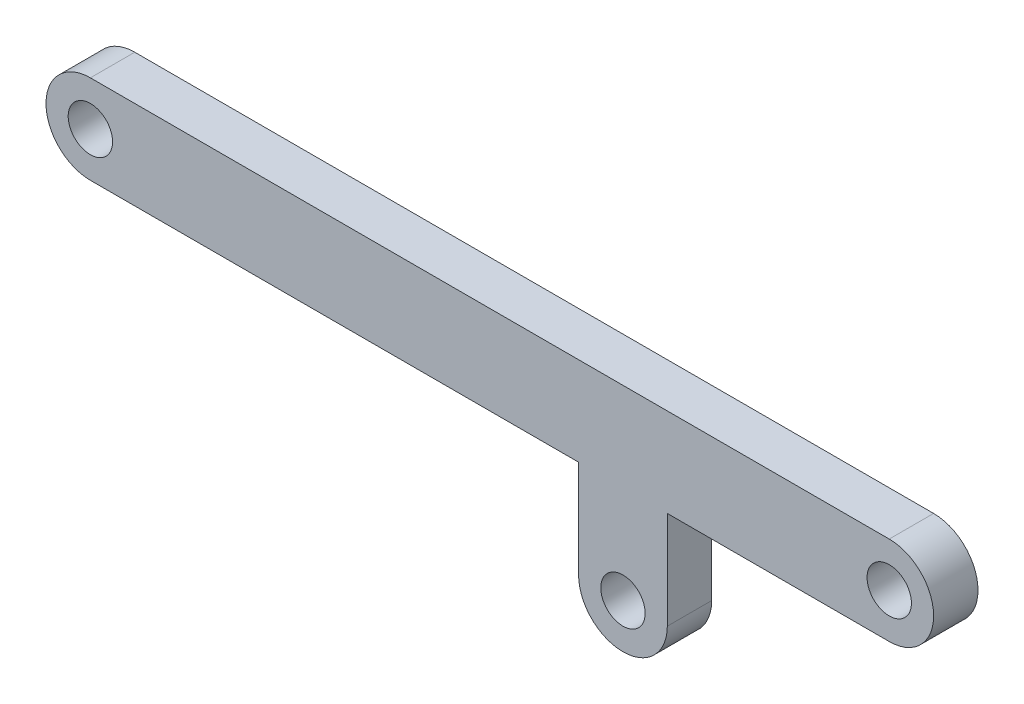
SolidWorks part; units mm, degrees
material "Plain Carbon Steel"
ref_plane "Front Plane" through (0, 0, 0) normal (0, 0, 1) x (1, 0, 0)
ref_plane "Top Plane" through (0, 0, 0) normal (0, 1, 0) x (1, 0, 0)
ref_plane "Right Plane" through (0, 0, 0) normal (1, 0, 0) x (0, 0, -1)
sketch "Link Plate Profile" plane through (0, 0, 0) normal (0, 0, 1) x (1, 0, 0)
  line L0 (45, 0) -> (-45, 0) construction
  line L1 (45, -5) -> (-45, -5)
  line L2 (45, 5) -> (-45, 5)
  line L3 (15, 6) -> (15, -16) construction
  line L4 (20, 6) -> (20, -16)
  line L5 (10, 6) -> (10, -16)
  arc A0 (45, -5) -> (45, 5) centre (45, 0) ccw
  arc A1 (-45, 5) -> (-45, -5) centre (-45, 0) ccw
  arc A2 (20, 6) -> (10, 6) centre (15, 6) ccw
  arc A3 (10, -16) -> (20, -16) centre (15, -16) ccw
  circle A4 centre (-45, 0) radius 2.5
  circle A5 centre (45, 0) radius 2.5
  circle A6 centre (15, -16) radius 2.5
  point P2 (0, 0)
  point P9 (15, -5)
  dimension "D1" = 5
  dimension "D2" = 5
  dimension "D5" = 5
  dimension "D3" = 90
  dimension "D4" = 30
  dimension "D6" = 11
extrude "Link Plate 5mm" add sketch "Link Plate Profile" along normal mid plane 5 contours L2 A1 L1 L5 A4 | L2 L5 L1 L4 | L1 A0 L2 L4 A5 | L5 A3 L4 L1 A6
